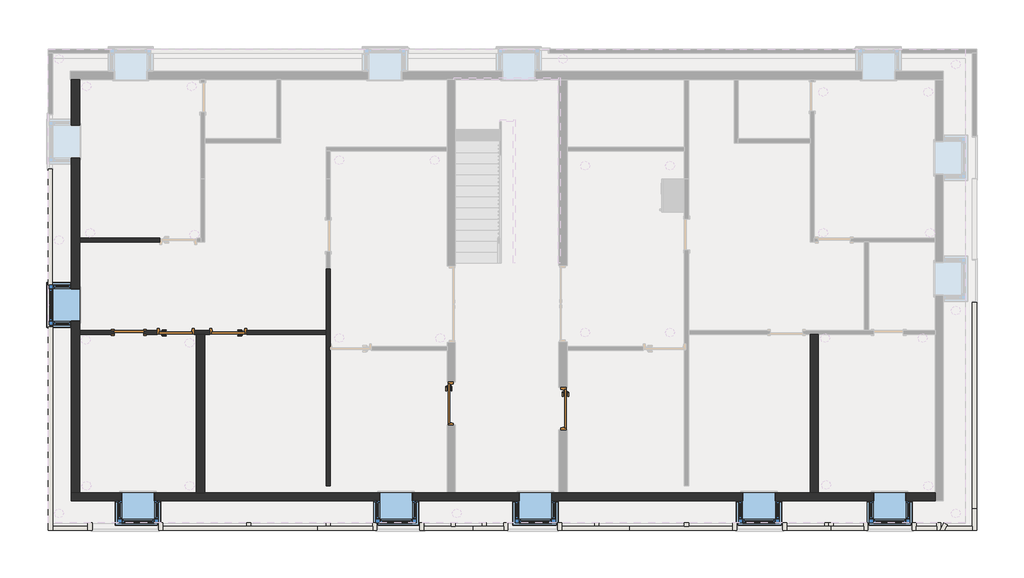
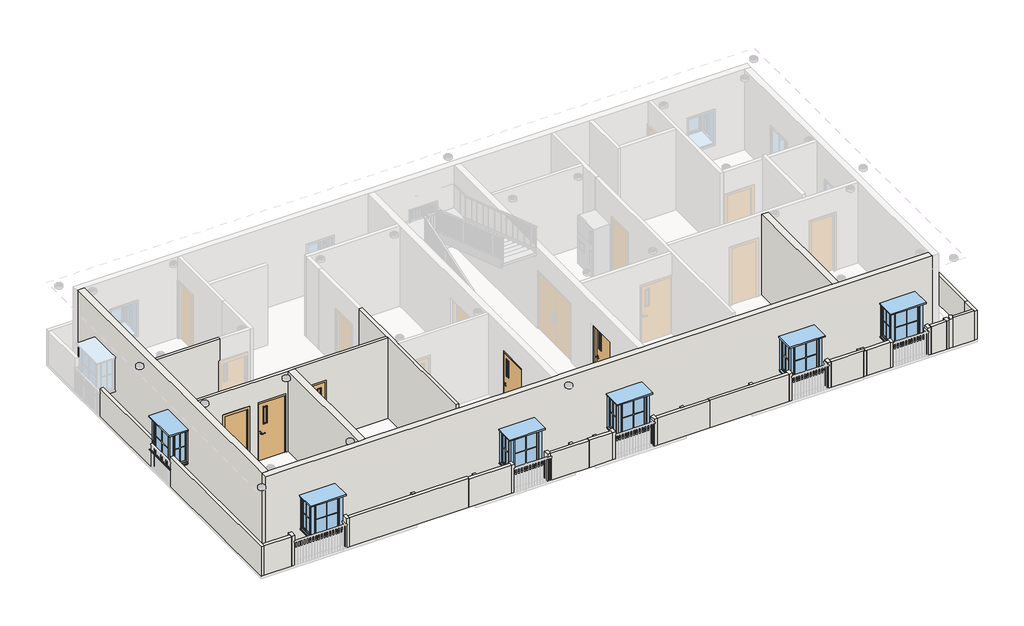
# One storey, part 1 of 7: 42 walls, 6 windows, 5 doors.
"""IFC4 building model written with IfcOpenShell, lengths in millimetres."""

from ifc_helpers import new_model, si_unit, frame, origin, place, context, project, spatial, polyline, outline, extrude, faceted_brep, transform, mapped, element, save
from components import door_586e558e, door_7d8f8091, door_passage_single_vision_lite_3_x7_440dd290, door_passage_single_vision_lite_3_x7_38248cdf, door_d141acb4, window_bay_casement_box_90_degree_angle_center_fixed_4_x3_2dea7aab

model = new_model("IFC4")

# Units and contexts
model_context = context("Model", 3, world=origin())
ifc_project = project(units=[si_unit("LENGTHUNIT", "METRE", prefix="MILLI")], contexts=[model_context])

# Site, building, storey
site = spatial("IfcSite", under=ifc_project)
building = spatial("IfcBuilding", under=site)
storey = spatial("IfcBuildingStorey", under=building, Elevation=3200.4)

# Doors
placement = place(None, origin())
door_shape = door_586e558e(model_context)
element("IfcDoor", 1, ObjectType="Door-Passage-Single-Vision_Lite : 3'6\"X7' 2", at=placement, inside=storey, context=model_context, shape_type="MappedRepresentation", body=[
    mapped(door_shape, transform((1116.1432011, -1461.3932193, 3200.4), x_axis=(0.0, -1.0, 0.0), y_axis=(1.0, 0.0, 0.0), z_axis=(0.0, 0.0, 1.0))),
])
door_2_shape = door_7d8f8091(model_context)
element("IfcDoor", 2, ObjectType="Door-Passage-Single-Vision_Lite : 3'7\"X7' 3", at=placement, inside=storey, context=model_context, shape_type="MappedRepresentation", body=[
    mapped(door_2_shape, transform((-1956.7487998, -1318.7421379, 3200.4), x_axis=(0.0, -1.0, 0.0), y_axis=(1.0, 0.0, 0.0), z_axis=(0.0, 0.0, 1.0))),
])
door_passage_single_vision_lite_3_x7_shape = door_passage_single_vision_lite_3_x7_440dd290(model_context)
element("IfcDoor", 3, ObjectType="Door-Passage-Single-Vision_Lite : 3'X7'", at=placement, inside=storey, context=model_context, shape_type="MappedRepresentation", body=[
    mapped(door_passage_single_vision_lite_3_x7_shape, transform((-8122.5987992, 646.8067334, 3200.4), x_axis=(-1.0, 0.0, 0.0), y_axis=(0.0, -1.0, 0.0), z_axis=(0.0, 0.0, 1.0))),
])
door_passage_single_vision_lite_3_x7_2_shape = door_passage_single_vision_lite_3_x7_38248cdf(model_context)
element("IfcDoor", 4, ObjectType="Door-Passage-Single-Vision_Lite : 3'X7'", at=placement, inside=storey, context=model_context, shape_type="MappedRepresentation", body=[
    mapped(door_passage_single_vision_lite_3_x7_2_shape, transform((-9570.3987992, 646.8067334, 3200.4), x_axis=(1.0, 0.0, 0.0), y_axis=(0.0, 1.0, 0.0), z_axis=(0.0, 0.0, 1.0))),
])
door_3_shape = door_d141acb4(model_context)
element("IfcDoor", 5, ObjectType="Single-Flush : 2'8\"x 7'", at=placement, inside=storey, context=model_context, shape_type="MappedRepresentation", body=[
    mapped(door_3_shape, transform((-10865.7987992, 640.4567334, 3200.4), x_axis=(1.0, 0.0, 0.0), y_axis=(0.0, 1.0, 0.0), z_axis=(0.0, 0.0, 1.0))),
])

# Walls
element("IfcWall", 6, ObjectType="Generic - 4.5\"", at=placement, inside=storey, context=model_context, shape_type="SweptSolid", body=[
    extrude(outline(polyline([(6248.4, -9959.0462614), (6248.4, -12224.6987925), (3200.4, -12224.6987925), (3200.4, -10009.8462614), (5435.6, -10009.8462614), (5435.6, -9959.0462614), (6248.4, -9959.0462614)])), frame((0.0, 3136.0067332, 0.0), z_axis=(0.0, 1.0, 0.0), x_axis=(0.0, 0.0, 1.0)), (0.0, 0.0, 1.0), 114.3),
])
element("IfcWall", 7, ObjectType="Generic - 4.5\"", at=placement, inside=storey, context=model_context, shape_type="Brep", body=[
    faceted_brep([(-10459.3987992, 583.3067334, 5334.0), (-10459.3987992, 583.3067334, 3200.4), (-10078.3987992, 583.3067334, 3200.4), (-10078.3987992, 583.3067334, 5435.6), (-9062.3987992, 583.3067334, 5435.6), (-9062.3987992, 583.3067334, 3200.4), (-8998.8987992, 583.3067334, 3200.4), (-8770.2987992, 583.3067334, 3200.4), (-8630.5987992, 583.3067334, 3200.4), (-8630.5987992, 583.3067334, 5435.6), (-7614.5987992, 583.3067334, 5435.6), (-7614.5987992, 583.3067334, 3200.4), (-5417.4987995, 583.3067334, 3200.4), (-5417.4987995, 583.3067334, 6248.4), (-8770.2987992, 583.3067334, 6248.4), (-8998.8987992, 583.3067334, 6248.4), (-12224.6987925, 583.3067334, 6248.4), (-12224.6987925, 583.3067334, 3200.4), (-11272.1987992, 583.3067334, 3200.4), (-11272.1987992, 583.3067334, 5334.0), (-10078.3987992, 697.6067334, 3200.4), (-10459.3987992, 697.6067334, 3200.4), (-10459.3987992, 697.6067334, 5334.0), (-11272.1987992, 697.6067334, 5334.0), (-11272.1987992, 697.6067334, 3200.4), (-12224.6987925, 697.6067334, 3200.4), (-12224.6987925, 697.6067334, 6248.4), (-5417.4987995, 697.6067334, 6248.4), (-5417.4987995, 697.6067334, 3200.4), (-7614.5987992, 697.6067334, 3200.4), (-7614.5987992, 697.6067334, 5435.6), (-8630.5987992, 697.6067334, 5435.6), (-8630.5987992, 697.6067334, 3200.4), (-9062.3987992, 697.6067334, 3200.4), (-9062.3987992, 697.6067334, 5435.6), (-10078.3987992, 697.6067334, 5435.6)], [[[0, 1, 2, 3, 4, 5, 6, 7, 8, 9, 10, 11, 12, 13, 14, 15, 16, 17, 18, 19]], [[20, 21, 22, 23, 24, 25, 26, 27, 28, 29, 30, 31, 32, 33, 34, 35]], [[28, 12, 11, 29]], [[32, 8, 7, 6, 5, 33]], [[18, 17, 25, 24]], [[2, 1, 21, 20]], [[16, 15, 14, 13, 27, 26]], [[17, 16, 26, 25]], [[13, 12, 28, 27]], [[9, 8, 32, 31]], [[10, 9, 31, 30]], [[11, 10, 30, 29]], [[4, 34, 33, 5]], [[34, 4, 3, 35]], [[35, 3, 2, 20]], [[22, 21, 1, 0]], [[23, 22, 0, 19]], [[24, 23, 19, 18]]]),
])
element("IfcWall", 8, ObjectType="Generic - 4.5\"", at=placement, inside=storey, context=model_context, shape_type="Brep", body=[
    faceted_brep([(-5417.4987995, 2399.4067802, 3200.4), (-5417.4987995, 697.6067334, 3200.4), (-5417.4987995, 583.3067334, 3200.4), (-5417.4987995, -3594.9932193, 3200.4), (-5417.4987995, -3594.9932193, 6248.4), (-5417.4987995, 583.3067334, 6248.4), (-5417.4987995, 697.6067334, 6248.4), (-5417.4987995, 2399.4067802, 6248.4), (-5303.1987995, -3594.9932193, 6248.4), (-5303.1987995, -3594.9932193, 3200.4), (-5303.1987995, 148.1078621, 3200.4), (-5303.1987995, 148.1078621, 5435.6), (-5303.1987995, 262.4078621, 5435.6), (-5303.1987995, 262.4078621, 3200.4), (-5303.1987995, 2399.4067802, 3200.4), (-5303.1987995, 2399.4067802, 6248.4), (-5303.1987995, 262.4078621, 6248.4), (-5303.1987995, 148.1078621, 6248.4), (-5334.9487995, 262.4078621, 3200.4), (-5334.9487995, 148.1078621, 3200.4), (-5334.9487995, 262.4078621, 5435.6), (-5334.9487995, 148.1078621, 5435.6)], [[[0, 1, 2, 3, 4, 5, 6, 7]], [[8, 9, 10, 11, 12, 13, 14, 15, 16, 17]], [[3, 2, 1, 0, 14, 13, 18, 19, 10, 9]], [[4, 3, 9, 8]], [[7, 6, 5, 4, 8, 17, 16, 15]], [[0, 7, 15, 14]], [[20, 18, 13, 12]], [[19, 21, 11, 10]], [[21, 20, 12, 11]], [[18, 20, 21, 19]]]),
])
element("IfcWall", 9, ObjectType="Generic - 4.5\"", at=placement, inside=storey, context=model_context, shape_type="SweptSolid", body=[
    extrude(outline(polyline([(-11996.6067989, -4826.8932661), (-12974.5067989, -4826.8932661), (-12974.5067989, -4712.5932661), (-11996.6067989, -4712.5932661), (-11996.6067989, -4826.8932661)])), frame((0.0, 0.0, 3200.4), z_axis=(0.0, 0.0, 1.0), x_axis=(1.0, 0.0, 0.0)), (0.0, 0.0, 1.0), 1112.9417562),
])
element("IfcWall", 10, ObjectType="Generic - 4.5\"", at=placement, inside=storey, context=model_context, shape_type="Brep", body=[
    faceted_brep([(-13088.8067989, 792.8567339, 3200.4), (-13088.8067989, -4826.8932661, 3200.4), (-13088.8067989, -4826.8932661, 4314.567936), (-13088.8067989, 792.8567339, 4314.567936), (-12974.5067989, 792.8567339, 3200.4), (-12974.5067989, 792.8567339, 4314.567936), (-12974.5067989, -4826.8932661, 4314.567936), (-12974.5067989, -4826.8932661, 4313.3417562), (-12974.5067989, -4826.8932661, 3200.4), (-12974.5067989, -4712.5932661, 3200.4)], [[[0, 1, 2, 3]], [[4, 5, 6, 7, 8, 9]], [[1, 0, 4, 9, 8]], [[3, 2, 6, 5]], [[0, 3, 5, 4]], [[2, 1, 8, 7, 6]]]),
])
element("IfcWall", 11, ObjectType="Generic - 4.5\"", at=placement, inside=storey, context=model_context, shape_type="Brep", body=[
    faceted_brep([(-11996.6067989, -4623.6932193, 3200.4), (-11996.6067989, -4712.5932661, 3200.4), (-11996.6067989, -4826.8932661, 3200.4), (-11996.6067989, -4826.8932661, 4313.3417562), (-11996.6067989, -4826.8932661, 4334.3303619), (-11996.6067989, -4623.6932193, 4334.3303619), (-11882.3067989, -4623.6932193, 3200.4), (-11882.3067989, -4623.6932193, 4334.3303619), (-11882.3067989, -4826.8932661, 4334.3303619), (-11882.3067989, -4826.8932661, 3200.4)], [[[0, 1, 2, 3, 4, 5]], [[6, 7, 8, 9]], [[2, 1, 0, 6, 9]], [[5, 4, 8, 7]], [[0, 5, 7, 6]], [[4, 3, 2, 9, 8]]]),
])
element("IfcWall", 12, ObjectType="Generic - 4.5\"", at=placement, inside=storey, context=model_context, shape_type="Brep", body=[
    faceted_brep([(11660.3143245, -4826.8932661, 3200.4), (12426.0012043, -4826.8932661, 3200.4), (12426.0012043, -4826.8932661, 4292.2617784), (12426.0012043, -4826.8932661, 4303.5196614), (11660.3143245, -4826.8932661, 4303.5196614), (11660.3143245, -4826.8932661, 4289.9342527), (11716.0621594, -4712.5932661, 3200.4), (11716.0621594, -4712.5932661, 4303.5196614), (12426.0012043, -4712.5932661, 4303.5196614), (12426.0012043, -4712.5932661, 3200.4)], [[[0, 1, 2, 3, 4, 5]], [[6, 7, 8, 9]], [[1, 0, 6, 9]], [[4, 3, 8, 7]], [[3, 2, 1, 9, 8]], [[0, 5, 4, 7, 6]]]),
])
element("IfcWall", 13, ObjectType="Generic - 4.5\"", at=placement, inside=storey, context=model_context, shape_type="Brep", body=[
    faceted_brep([(11632.2512075, -4623.6932193, 3200.4), (11533.1439227, -4826.8932661, 3200.4), (11533.1439227, -4826.8932661, 4289.9342527), (11632.2512075, -4623.6932193, 4289.9342527), (11734.983367, -4673.7990414, 3200.4), (11734.983367, -4673.7990414, 4289.9342527), (11660.3143245, -4826.8932661, 4289.9342527), (11660.3143245, -4826.8932661, 3200.4), (11716.0621594, -4712.5932661, 3200.4)], [[[0, 1, 2, 3]], [[4, 5, 6, 7, 8]], [[1, 0, 4, 8, 7]], [[3, 2, 6, 5]], [[0, 3, 5, 4]], [[2, 1, 7, 6]]]),
])
element("IfcWall", 14, ObjectType="Generic - 4.5\"", at=placement, inside=storey, context=model_context, shape_type="Brep", body=[
    faceted_brep([(12426.0012043, -4236.3432661, 3200.4), (12426.0012043, -4712.5932661, 3200.4), (12426.0012043, -4826.8932661, 3200.4), (12426.0012043, -4826.8932661, 4292.2617784), (12426.0012043, -4236.3432661, 4292.2617784), (12426.0012043, -4236.3432661, 4287.0712164), (12540.3012043, -4236.3432661, 3200.4), (12540.3012043, -4236.3432661, 4287.0712164), (12540.3012043, -4236.3432661, 4292.2617784), (12540.3012043, -4826.8932661, 4292.2617784), (12540.3012043, -4826.8932661, 3200.4)], [[[0, 1, 2, 3, 4, 5]], [[6, 7, 8, 9, 10]], [[2, 1, 0, 6, 10]], [[4, 3, 9, 8]], [[0, 5, 4, 8, 7, 6]], [[3, 2, 10, 9]]]),
])
element("IfcWall", 15, ObjectType="Generic - 4.5\"", at=placement, inside=storey, context=model_context, shape_type="SweptSolid", body=[
    extrude(outline(polyline([(-5417.4987995, -4712.5932661), (-5417.4987995, -4623.6932193), (-5303.1987995, -4623.6932193), (-5303.1987995, -4712.5932661), (-5417.4987995, -4712.5932661)])), frame((0.0, 0.0, 3200.4), z_axis=(0.0, 0.0, 1.0), x_axis=(1.0, 0.0, 0.0)), (0.0, 0.0, 1.0), 1063.0786215),
])
element("IfcWall", 16, ObjectType="Generic - 4.5\"", at=placement, inside=storey, context=model_context, shape_type="Brep", body=[
    faceted_brep([(-5663.8033402, -4826.8932661, 3200.4), (-4134.7987995, -4826.8932661, 3200.4), (-4134.7987995, -4826.8932661, 4259.5218247), (-4134.7987995, -4826.8932661, 4267.6575049), (-5663.8033402, -4826.8932661, 4267.6575049), (-5663.8033402, -4712.5932661, 3200.4), (-5663.8033402, -4712.5932661, 4267.6575049), (-4134.7987995, -4712.5932661, 4267.6575049), (-4134.7987995, -4712.5932661, 3200.4), (-5303.1987995, -4712.5932661, 3200.4), (-5417.4987995, -4712.5932661, 3200.4)], [[[0, 1, 2, 3, 4]], [[5, 6, 7, 8, 9, 10]], [[1, 0, 5, 10, 9, 8]], [[4, 3, 7, 6]], [[0, 4, 6, 5]], [[3, 2, 1, 8, 7]]]),
])
element("IfcWall", 17, ObjectType="Generic - 4.5\"", at=placement, inside=storey, context=model_context, shape_type="Brep", body=[
    faceted_brep([(-2725.0987995, -4826.8932661, 3200.4), (-1354.4417672, -4826.8932661, 3200.4), (-1354.4417672, -4826.8932661, 4216.4), (-2725.0987995, -4826.8932661, 4216.4), (-2725.0987995, -4712.5932661, 3200.4), (-2725.0987995, -4712.5932661, 4216.4), (-1354.4417672, -4712.5932661, 4216.4), (-1354.4417672, -4712.5932661, 3200.4), (-1848.7987998, -4712.5932661, 3200.4), (-1963.0987998, -4712.5932661, 3200.4)], [[[0, 1, 2, 3]], [[4, 5, 6, 7, 8, 9]], [[1, 0, 4, 9, 8, 7]], [[2, 1, 7, 6]], [[3, 2, 6, 5]], [[0, 3, 5, 4]]]),
])
element("IfcWall", 18, ObjectType="Generic - 4.5\"", at=placement, inside=storey, context=model_context, shape_type="SweptSolid", body=[
    extrude(outline(polyline([(-1963.0987998, -4712.5932661), (-1963.0987998, -4623.6932193), (-1848.7987998, -4623.6932193), (-1848.7987998, -4712.5932661), (-1963.0987998, -4712.5932661)])), frame((0.0, 0.0, 3200.4), z_axis=(0.0, 0.0, 1.0), x_axis=(1.0, 0.0, 0.0)), (0.0, 0.0, 1.0), 1029.3234006),
])
element("IfcWall", 19, ObjectType="Generic - 4.5\"", at=placement, inside=storey, context=model_context, shape_type="SweptSolid", body=[
    extrude(outline(polyline([(-1112.1987998, -4712.5932661), (-1112.1987998, -4623.6932193), (-997.8987998, -4623.6932193), (-997.8987998, -4712.5932661), (-1112.1987998, -4712.5932661)])), frame((0.0, 0.0, 3200.4), z_axis=(0.0, 0.0, 1.0), x_axis=(1.0, 0.0, 0.0)), (0.0, 0.0, 1.0), 1016.0),
])
element("IfcWall", 20, ObjectType="Generic - 4.5\"", at=placement, inside=storey, context=model_context, shape_type="SweptSolid", body=[
    extrude(outline(polyline([(1999.3012002, -4712.5932661), (1999.3012002, -4623.6932193), (2113.6012002, -4623.6932193), (2113.6012002, -4712.5932661), (1999.3012002, -4712.5932661)])), frame((0.0, 0.0, 3200.4), z_axis=(0.0, 0.0, 1.0), x_axis=(1.0, 0.0, 0.0)), (0.0, 0.0, 1.0), 1013.2250283),
])
element("IfcWall", 21, ObjectType="Generic - 4.5\"", at=placement, inside=storey, context=model_context, shape_type="SweptSolid", body=[
    extrude(outline(polyline([(4475.8012082, -4712.5932661), (4475.8012082, -4623.6932193), (4590.1012082, -4623.6932193), (4590.1012082, -4712.5932661), (4475.8012082, -4712.5932661)])), frame((0.0, 0.0, 3200.4), z_axis=(0.0, 0.0, 1.0), x_axis=(1.0, 0.0, 0.0)), (0.0, 0.0, 1.0), 1027.4591445),
])
element("IfcWall", 22, ObjectType="Generic - 4.5\"", at=placement, inside=storey, context=model_context, shape_type="Brep", body=[
    faceted_brep([(2962.6087812, -4826.8932661, 3200.4), (5802.9512082, -4826.8932661, 3200.4), (5802.9512082, -4826.8932661, 4227.8591445), (2962.6087812, -4826.8932661, 4227.8591445), (2962.6087812, -4826.8932661, 4213.6250283), (2962.6087812, -4712.5932661, 3200.4), (2962.6087812, -4712.5932661, 4213.6250283), (2962.6087812, -4712.5932661, 4227.8591445), (4475.8012082, -4712.5932661, 4227.8591445), (4590.1012082, -4712.5932661, 4227.8591445), (5802.9512082, -4712.5932661, 4227.8591445), (5802.9512082, -4712.5932661, 3200.4), (4590.1012082, -4712.5932661, 3200.4), (4475.8012082, -4712.5932661, 3200.4)], [[[0, 1, 2, 3, 4]], [[5, 6, 7, 8, 9, 10, 11, 12, 13]], [[1, 0, 5, 13, 12, 11]], [[3, 2, 10, 9, 8, 7]], [[0, 4, 3, 7, 6, 5]], [[2, 1, 11, 10]]]),
])
element("IfcWall", 23, ObjectType="Generic - 4.5\"", at=placement, inside=storey, context=model_context, shape_type="Brep", body=[
    faceted_brep([(5802.9512082, -4623.6932193, 3200.4), (5802.9512082, -4712.5932661, 3200.4), (5802.9512082, -4826.8932661, 3200.4), (5802.9512082, -4826.8932661, 4227.8591445), (5802.9512082, -4826.8932661, 4232.7822201), (5802.9512082, -4623.6932193, 4232.7822201), (5917.2512082, -4623.6932193, 3200.4), (5917.2512082, -4623.6932193, 4232.7822201), (5917.2512082, -4826.8932661, 4232.7822201), (5917.2512082, -4826.8932661, 3200.4)], [[[0, 1, 2, 3, 4, 5]], [[6, 7, 8, 9]], [[2, 1, 0, 6, 9]], [[5, 4, 8, 7]], [[0, 5, 7, 6]], [[4, 3, 2, 9, 8]]]),
])
element("IfcWall", 24, ObjectType="Generic - 4.5\"", at=placement, inside=storey, context=model_context, shape_type="Brep", body=[
    faceted_brep([(7190.3011643, -4623.6932193, 3200.4), (7190.3011643, -4826.8932661, 3200.4), (7190.3011643, -4826.8932661, 4173.2158009), (7190.3011643, -4623.6932193, 4173.2158009), (7304.6011643, -4623.6932193, 3200.4), (7304.6011643, -4623.6932193, 4173.2158009), (7304.6011643, -4712.5932661, 4173.2158009), (7304.6011643, -4826.8932661, 4173.2158009), (7304.6011643, -4826.8932661, 3200.4), (7304.6011643, -4712.5932661, 3200.4)], [[[0, 1, 2, 3]], [[4, 5, 6, 7, 8, 9]], [[1, 0, 4, 9, 8]], [[3, 2, 7, 6, 5]], [[0, 3, 5, 4]], [[2, 1, 8, 7]]]),
])
element("IfcWall", 25, ObjectType="Generic - 4.5\"", at=placement, inside=storey, context=model_context, shape_type="Brep", body=[
    faceted_brep([(7304.6011643, -4826.8932661, 3200.4), (8463.6012082, -4826.8932661, 3200.4), (8463.6012082, -4826.8932661, 4156.8159658), (8520.7512082, -4826.8932661, 4156.8159658), (8520.7512082, -4826.8932661, 4170.080309), (8520.7512082, -4826.8932661, 4173.3581334), (7304.6011643, -4826.8932661, 4173.3581334), (7304.6011643, -4712.5932661, 3200.4), (7304.6011643, -4712.5932661, 4173.3581334), (8520.7512082, -4712.5932661, 4173.3581334), (8520.7512082, -4712.5932661, 4170.080309), (8520.7512082, -4712.5932661, 4156.8159658), (8463.6012082, -4712.5932661, 4156.8159658), (8463.6012082, -4712.5932661, 3200.4), (8457.2512082, -4712.5932661, 3200.4), (8342.9512082, -4712.5932661, 3200.4)], [[[0, 1, 2, 3, 4, 5, 6]], [[7, 8, 9, 10, 11, 12, 13, 14, 15]], [[1, 0, 7, 15, 14, 13]], [[6, 5, 9, 8]], [[0, 6, 8, 7]], [[5, 4, 3, 11, 10, 9]], [[11, 3, 2, 12]], [[2, 1, 13, 12]]]),
])
element("IfcWall", 26, ObjectType="Generic - 4.5\"", at=placement, inside=storey, context=model_context, shape_type="SweptSolid", body=[
    extrude(outline(polyline([(8342.9512082, -4712.5932661), (8342.9512082, -4623.6932193), (8457.2512082, -4623.6932193), (8457.2512082, -4712.5932661), (8342.9512082, -4712.5932661)])), frame((0.0, 0.0, 3200.4), z_axis=(0.0, 0.0, 1.0), x_axis=(1.0, 0.0, 0.0)), (0.0, 0.0, 1.0), 954.7500484),
])
element("IfcWall", 27, ObjectType="Generic - 4.5\"", at=placement, inside=storey, context=model_context, shape_type="Brep", body=[
    faceted_brep([(8463.6012082, -4623.6932193, 3200.4), (8463.6012082, -4712.5932661, 3200.4), (8463.6012082, -4826.8932661, 3200.4), (8463.6012082, -4826.8932661, 4156.8159658), (8463.6012082, -4712.5932661, 4156.8159658), (8463.6012082, -4623.6932193, 4156.8159658), (8577.9012082, -4623.6932193, 3200.4), (8577.9012082, -4623.6932193, 4156.8159658), (8577.9012082, -4712.5932661, 4156.8159658), (8577.9012082, -4826.8932661, 4156.8159658), (8577.9012082, -4826.8932661, 3200.4), (8577.9012082, -4712.5932661, 3200.4), (8520.7512082, -4826.8932661, 4156.8159658)], [[[0, 1, 2, 3, 4, 5]], [[6, 7, 8, 9, 10, 11]], [[2, 1, 0, 6, 11, 10]], [[5, 4, 3, 12, 9, 8, 7]], [[0, 5, 7, 6]], [[3, 2, 10, 9, 12]]]),
])
element("IfcWall", 28, ObjectType="Generic - 4.5\"", at=placement, inside=storey, context=model_context, shape_type="Brep", body=[
    faceted_brep([(8577.9012082, -4826.8932661, 3200.4), (9422.4512082, -4826.8932661, 3200.4), (9422.4512082, -4826.8932661, 4152.6060641), (9422.4512082, -4826.8932661, 4170.080309), (8520.7512082, -4826.8932661, 4170.080309), (8520.7512082, -4826.8932661, 4156.8159658), (8577.9012082, -4826.8932661, 4156.8159658), (8577.9012082, -4712.5932661, 3200.4), (8577.9012082, -4712.5932661, 4156.8159658), (8520.7512082, -4712.5932661, 4156.8159658), (8520.7512082, -4712.5932661, 4170.080309), (9422.4512082, -4712.5932661, 4170.080309), (9422.4512082, -4712.5932661, 3200.4)], [[[0, 1, 2, 3, 4, 5, 6]], [[7, 8, 9, 10, 11, 12]], [[1, 0, 7, 12]], [[4, 3, 11, 10]], [[3, 2, 1, 12, 11]], [[5, 4, 10, 9]], [[5, 9, 8, 6]], [[0, 6, 8, 7]]]),
])
element("IfcWall", 29, ObjectType="Generic - 4.5\"", at=placement, inside=storey, context=model_context, shape_type="Brep", body=[
    faceted_brep([(9422.4512082, -4623.6932193, 3200.4), (9422.4512082, -4712.5932661, 3200.4), (9422.4512082, -4826.8932661, 3200.4), (9422.4512082, -4826.8932661, 4152.6060641), (9422.4512082, -4623.6932193, 4152.6060641), (9536.7512082, -4623.6932193, 3200.4), (9536.7512082, -4623.6932193, 4152.6060641), (9536.7512082, -4826.8932661, 4152.6060641), (9536.7512082, -4826.8932661, 3200.4)], [[[0, 1, 2, 3, 4]], [[5, 6, 7, 8]], [[2, 1, 0, 5, 8]], [[4, 3, 7, 6]], [[0, 4, 6, 5]], [[3, 2, 8, 7]]]),
])
element("IfcWall", 30, ObjectType="Generic - 4.5\"", at=placement, inside=storey, context=model_context, shape_type="Brep", body=[
    faceted_brep([(10764.1617205, -4623.6932193, 3200.4), (10764.1617205, -4826.8932661, 3200.4), (10764.1617205, -4826.8932661, 4226.7072304), (10764.1617205, -4623.6932193, 4226.7072304), (10878.4617205, -4623.6932193, 3200.4), (10878.4617205, -4623.6932193, 4226.7072304), (10878.4617205, -4826.8932661, 4226.7072304), (10878.4617205, -4826.8932661, 3200.4), (10878.4617205, -4712.5932661, 3200.4)], [[[0, 1, 2, 3]], [[4, 5, 6, 7, 8]], [[1, 0, 4, 8, 7]], [[3, 2, 6, 5]], [[0, 3, 5, 4]], [[2, 1, 7, 6]]]),
])
element("IfcWall", 31, ObjectType="Generic - 4.5\"", at=placement, inside=storey, context=model_context, shape_type="Brep", body=[
    faceted_brep([(10878.4617205, -4826.8932661, 3200.4), (11437.2617205, -4826.8932661, 3200.4), (11437.2617205, -4826.8932661, 4249.0912221), (10878.4617205, -4826.8932661, 4249.0912221), (10878.4617205, -4826.8932661, 4226.7072304), (10878.4617205, -4712.5932661, 3200.4), (10878.4617205, -4712.5932661, 4249.0912221), (11437.2617205, -4712.5932661, 4249.0912221), (11437.2617205, -4712.5932661, 3200.4)], [[[0, 1, 2, 3, 4]], [[5, 6, 7, 8]], [[1, 0, 5, 8]], [[3, 2, 7, 6]], [[0, 4, 3, 6, 5]], [[2, 1, 8, 7]]]),
])
element("IfcWall", 32, ObjectType="Generic - 4.5\"", at=placement, inside=storey, context=model_context, shape_type="Brep", body=[
    faceted_brep([(11437.2617205, -4623.6932193, 3200.4), (11437.2617205, -4712.5932661, 3200.4), (11437.2617205, -4826.8932661, 3200.4), (11437.2617205, -4826.8932661, 4249.0912221), (11437.2617205, -4712.5932661, 4249.0912221), (11437.2617205, -4623.6932193, 4249.0912221), (11551.5617205, -4623.6932193, 3200.4), (11551.5617205, -4623.6932193, 4249.0912221), (11551.5617205, -4826.8932661, 4249.0912221), (11551.5617205, -4826.8932661, 3200.4)], [[[0, 1, 2, 3, 4, 5]], [[6, 7, 8, 9]], [[2, 1, 0, 6, 9]], [[5, 4, 3, 8, 7]], [[0, 5, 7, 6]], [[3, 2, 9, 8]]]),
])
element("IfcWall", 33, ObjectType="Generic - 4.5\"", at=placement, inside=storey, context=model_context, shape_type="Brep", body=[
    faceted_brep([(-4134.7987995, -4623.6932193, 3200.4), (-4134.7987995, -4712.5932661, 3200.4), (-4134.7987995, -4826.8932661, 3200.4), (-4134.7987995, -4826.8932661, 4259.5218247), (-4134.7987995, -4623.6932193, 4259.5218247), (-4020.4987995, -4623.6932193, 3200.4), (-4020.4987995, -4623.6932193, 4259.5218247), (-4020.4987995, -4826.8932661, 4259.5218247), (-4020.4987995, -4826.8932661, 3200.4)], [[[0, 1, 2, 3, 4]], [[5, 6, 7, 8]], [[2, 1, 0, 5, 8]], [[4, 3, 7, 6]], [[0, 4, 6, 5]], [[3, 2, 8, 7]]]),
])
element("IfcWall", 34, ObjectType="Generic - 4.5\"", at=placement, inside=storey, context=model_context, shape_type="Brep", body=[
    faceted_brep([(-2839.3987995, -4623.6932193, 3200.4), (-2839.3987995, -4826.8932661, 3200.4), (-2839.3987995, -4826.8932661, 4217.1549618), (-2839.3987995, -4623.6932193, 4217.1549618), (-2725.0987995, -4623.6932193, 3200.4), (-2725.0987995, -4623.6932193, 4217.1549618), (-2725.0987995, -4826.8932661, 4217.1549618), (-2725.0987995, -4826.8932661, 4216.4), (-2725.0987995, -4826.8932661, 3200.4), (-2725.0987995, -4712.5932661, 3200.4)], [[[0, 1, 2, 3]], [[4, 5, 6, 7, 8, 9]], [[1, 0, 4, 9, 8]], [[3, 2, 6, 5]], [[0, 3, 5, 4]], [[2, 1, 8, 7, 6]]]),
])
element("IfcWall", 35, ObjectType="Generic - 4.5\"", at=placement, inside=storey, context=model_context, shape_type="Brep", body=[
    faceted_brep([(-1354.4417672, -4826.8932661, 3200.4), (-520.5065315, -4826.8932661, 3200.4), (-520.5065315, -4826.8932661, 4224.2796817), (-520.5065315, -4826.8932661, 4231.540074), (-1354.4417672, -4826.8932661, 4231.540074), (-1354.4417672, -4826.8932661, 4216.4), (-1354.4417672, -4712.5932661, 3200.4), (-1354.4417672, -4712.5932661, 4216.4), (-1354.4417672, -4712.5932661, 4231.540074), (-520.5065315, -4712.5932661, 4231.540074), (-520.5065315, -4712.5932661, 3200.4), (-997.8987998, -4712.5932661, 3200.4), (-1112.1987998, -4712.5932661, 3200.4)], [[[0, 1, 2, 3, 4, 5]], [[6, 7, 8, 9, 10, 11, 12]], [[1, 0, 6, 12, 11, 10]], [[4, 3, 9, 8]], [[0, 5, 4, 8, 7, 6]], [[3, 2, 1, 10, 9]]]),
])
element("IfcWall", 36, ObjectType="Generic - 4.5\"", at=placement, inside=storey, context=model_context, shape_type="Brep", body=[
    faceted_brep([(-520.5065315, -4623.6932193, 3200.4), (-520.5065315, -4712.5932661, 3200.4), (-520.5065315, -4826.8932661, 3200.4), (-520.5065315, -4826.8932661, 4224.2796817), (-520.5065315, -4623.6932193, 4224.2796817), (-406.2065315, -4623.6932193, 3200.4), (-406.2065315, -4623.6932193, 4224.2796817), (-406.2065315, -4826.8932661, 4224.2796817), (-406.2065315, -4826.8932661, 3200.4)], [[[0, 1, 2, 3, 4]], [[5, 6, 7, 8]], [[2, 1, 0, 5, 8]], [[4, 3, 7, 6]], [[0, 4, 6, 5]], [[3, 2, 8, 7]]]),
])
element("IfcWall", 37, ObjectType="Generic - 4.5\"", at=placement, inside=storey, context=model_context, shape_type="Brep", body=[
    faceted_brep([(970.0932011, -4623.6932193, 3200.4), (970.0932011, -4826.8932661, 3200.4), (970.0932011, -4826.8932661, 4213.6250283), (970.0932011, -4623.6932193, 4213.6250283), (1084.3932011, -4623.6932193, 3200.4), (1084.3932011, -4623.6932193, 4213.6250283), (1084.3932011, -4712.5932661, 4213.6250283), (1084.3932011, -4826.8932661, 4213.6250283), (1084.3932011, -4826.8932661, 3200.4), (1084.3932011, -4712.5932661, 3200.4)], [[[0, 1, 2, 3]], [[4, 5, 6, 7, 8, 9]], [[1, 0, 4, 9, 8]], [[3, 2, 7, 6, 5]], [[0, 3, 5, 4]], [[2, 1, 8, 7]]]),
])
element("IfcWall", 38, ObjectType="Generic - 4.5\"", at=placement, inside=storey, context=model_context, shape_type="Brep", body=[
    faceted_brep([(1084.3932011, -4826.8932661, 3200.4), (2962.6087812, -4826.8932661, 3200.4), (2962.6087812, -4826.8932661, 4213.6250283), (1084.3932011, -4826.8932661, 4213.6250283), (1084.3932011, -4712.5932661, 3200.4), (1084.3932011, -4712.5932661, 4213.6250283), (1999.3012002, -4712.5932661, 4213.6250283), (2113.6012002, -4712.5932661, 4213.6250283), (2962.6087812, -4712.5932661, 4213.6250283), (2962.6087812, -4712.5932661, 3200.4), (2113.6012002, -4712.5932661, 3200.4), (1999.3012002, -4712.5932661, 3200.4)], [[[0, 1, 2, 3]], [[4, 5, 6, 7, 8, 9, 10, 11]], [[1, 0, 4, 11, 10, 9]], [[2, 1, 9, 8]], [[3, 2, 8, 7, 6, 5]], [[0, 3, 5, 4]]]),
])
element("IfcWall", 39, ObjectType="Generic - 4.5\"", at=placement, inside=storey, context=model_context, shape_type="Brep", body=[
    faceted_brep([(-10045.9470335, -4623.6932193, 3200.4), (-10045.9470335, -4826.8932661, 3200.4), (-10045.9470335, -4826.8932661, 4308.104535), (-10045.9470335, -4623.6932193, 4308.104535), (-9931.6470335, -4623.6932193, 3200.4), (-9931.6470335, -4623.6932193, 4308.104535), (-9931.6470335, -4712.5932661, 4308.104535), (-9931.6470335, -4826.8932661, 4308.104535), (-9931.6470335, -4826.8932661, 3200.4), (-9931.6470335, -4712.5932661, 3200.4)], [[[0, 1, 2, 3]], [[4, 5, 6, 7, 8, 9]], [[1, 0, 4, 9, 8]], [[3, 2, 7, 6, 5]], [[0, 3, 5, 4]], [[2, 1, 8, 7]]]),
])
element("IfcWall", 40, ObjectType="Generic - 4.5\"", at=placement, inside=storey, context=model_context, shape_type="Brep", body=[
    faceted_brep([(-9931.6470335, -4826.8932661, 3200.4), (-5663.8033402, -4826.8932661, 3200.4), (-5663.8033402, -4826.8932661, 4267.6575049), (-5663.8033402, -4826.8932661, 4308.104535), (-9931.6470335, -4826.8932661, 4308.104535), (-9931.6470335, -4712.5932661, 3200.4), (-9931.6470335, -4712.5932661, 4308.104535), (-7614.8527957, -4712.5932661, 4308.104535), (-7500.5527957, -4712.5932661, 4308.104535), (-5663.8033402, -4712.5932661, 4308.104535), (-5663.8033402, -4712.5932661, 4267.6575049), (-5663.8033402, -4712.5932661, 3200.4), (-7500.5527957, -4712.5932661, 3200.4), (-7614.8527957, -4712.5932661, 3200.4)], [[[0, 1, 2, 3, 4]], [[5, 6, 7, 8, 9, 10, 11, 12, 13]], [[1, 0, 5, 13, 12, 11]], [[3, 2, 1, 11, 10, 9]], [[4, 3, 9, 8, 7, 6]], [[0, 4, 6, 5]]]),
])
element("IfcWall", 41, ObjectType="Generic - 4.5\"", at=placement, inside=storey, context=model_context, shape_type="SweptSolid", body=[
    extrude(outline(polyline([(-7614.8527957, -4712.5932661), (-7614.8527957, -4623.6932193), (-7500.5527957, -4623.6932193), (-7500.5527957, -4712.5932661), (-7614.8527957, -4712.5932661)])), frame((0.0, 0.0, 3200.4), z_axis=(0.0, 0.0, 1.0), x_axis=(1.0, 0.0, 0.0)), (0.0, 0.0, 1.0), 1107.704535),
])
element("IfcWall", 42, ObjectType="Generic - 4.5\"", at=placement, inside=storey, context=model_context, shape_type="SweptSolid", body=[
    extrude(outline(polyline([(-12976.0338648, 5154.3604213), (-12976.0338648, 1953.9604213), (-13090.3338648, 1953.9604213), (-13090.3338648, 5154.3604213), (-12976.0338648, 5154.3604213)])), frame((0.0, 0.0, 3200.4), z_axis=(0.0, 0.0, 1.0), x_axis=(1.0, 0.0, 0.0)), (0.0, 0.0, 1.0), 1047.4413329),
])
element("IfcWall", 43, ObjectType="Generic - 4.5\"", at=placement, inside=storey, context=model_context, shape_type="SweptSolid", body=[
    extrude(outline(polyline([(12426.0012043, -4236.3432661), (12426.0012043, 1478.6567334), (12540.3012043, 1478.6567334), (12540.3012043, -4236.3432661), (12426.0012043, -4236.3432661)])), frame((0.0, 0.0, 3200.4), z_axis=(0.0, 0.0, 1.0), x_axis=(1.0, 0.0, 0.0)), (0.0, 0.0, 1.0), 1086.6712164),
])
element("IfcWall", 44, ObjectType="Generic - 9\"", at=placement, inside=storey, context=model_context, shape_type="Brep", body=[
    faceted_brep([(11397.3012075, -3785.4932193, 3200.4), (8171.5012079, -3785.4932193, 3200.4), (7942.9012079, -3785.4932193, 3200.4), (1236.7932011, -3785.4932193, 3200.4), (1008.1932011, -3785.4932193, 3200.4), (-1848.7987998, -3785.4932193, 3200.4), (-2077.3987998, -3785.4932193, 3200.4), (-8770.2987992, -3785.4932193, 3200.4), (-8998.8987992, -3785.4932193, 3200.4), (-12224.6987925, -3785.4932193, 3200.4), (-12453.2987925, -3785.4932193, 3200.4), (-12453.2987925, -3785.4932193, 6248.4), (-12224.6987925, -3785.4932193, 6248.4), (-8998.8987992, -3785.4932193, 6248.4), (-8770.2987992, -3785.4932193, 6248.4), (-2077.3987998, -3785.4932193, 6248.4), (-1848.7987998, -3785.4932193, 6248.4), (1008.1932011, -3785.4932193, 6248.4), (1236.7932011, -3785.4932193, 6248.4), (7942.9012079, -3785.4932193, 6248.4), (8171.5012079, -3785.4932193, 6248.4), (11397.3012075, -3785.4932193, 6248.4), (-11068.9987958, -3785.4932193, 5080.0), (-11068.9987958, -3785.4932193, 3810.0), (-10154.5987958, -3785.4932193, 3810.0), (-10154.5987958, -3785.4932193, 5080.0), (-3944.2987998, -3785.4932193, 5080.0), (-3944.2987998, -3785.4932193, 3810.0), (-3029.8987998, -3785.4932193, 3810.0), (-3029.8987998, -3785.4932193, 5080.0), (-96.7067989, -3785.4932193, 5080.0), (-96.7067989, -3785.4932193, 3810.0), (817.6932011, -3785.4932193, 3810.0), (817.6932011, -3785.4932193, 5080.0), (6076.0012079, -3785.4932193, 5080.0), (6076.0012079, -3785.4932193, 3810.0), (6990.4012079, -3785.4932193, 3810.0), (6990.4012079, -3785.4932193, 5080.0), (9682.8012075, -3785.4932193, 5080.0), (9682.8012075, -3785.4932193, 3810.0), (10597.2012075, -3785.4932193, 3810.0), (10597.2012075, -3785.4932193, 5080.0), (11397.3012075, -4014.0932193, 3200.4), (11397.3012075, -4014.0932193, 6248.4), (-12453.2987925, -4014.0932193, 6248.4), (-12453.2987925, -4014.0932193, 3200.4), (-11068.9987958, -4014.0932193, 5080.0), (-10154.5987958, -4014.0932193, 5080.0), (-10154.5987958, -4014.0932193, 3810.0), (-11068.9987958, -4014.0932193, 3810.0), (-3944.2987998, -4014.0932193, 5080.0), (-3029.8987998, -4014.0932193, 5080.0), (-3029.8987998, -4014.0932193, 3810.0), (-3944.2987998, -4014.0932193, 3810.0), (-96.7067989, -4014.0932193, 5080.0), (817.6932011, -4014.0932193, 5080.0), (817.6932011, -4014.0932193, 3810.0), (-96.7067989, -4014.0932193, 3810.0), (6076.0012079, -4014.0932193, 5080.0), (6990.4012079, -4014.0932193, 5080.0), (6990.4012079, -4014.0932193, 3810.0), (6076.0012079, -4014.0932193, 3810.0), (9682.8012075, -4014.0932193, 5080.0), (10597.2012075, -4014.0932193, 5080.0), (10597.2012075, -4014.0932193, 3810.0), (9682.8012075, -4014.0932193, 3810.0)], [[[0, 1, 2, 3, 4, 5, 6, 7, 8, 9, 10, 11, 12, 13, 14, 15, 16, 17, 18, 19, 20, 21], [22, 23, 24, 25], [26, 27, 28, 29], [30, 31, 32, 33], [34, 35, 36, 37], [38, 39, 40, 41]], [[42, 43, 44, 45], [46, 47, 48, 49], [50, 51, 52, 53], [54, 55, 56, 57], [58, 59, 60, 61], [62, 63, 64, 65]], [[10, 9, 8, 7, 6, 5, 4, 3, 2, 1, 0, 42, 45]], [[21, 20, 19, 18, 17, 16, 15, 14, 13, 12, 11, 44, 43]], [[0, 21, 43, 42]], [[11, 10, 45, 44]], [[23, 22, 46, 49]], [[24, 23, 49, 48]], [[25, 24, 48, 47]], [[22, 25, 47, 46]], [[27, 26, 50, 53]], [[28, 27, 53, 52]], [[29, 28, 52, 51]], [[26, 29, 51, 50]], [[31, 30, 54, 57]], [[32, 31, 57, 56]], [[33, 32, 56, 55]], [[30, 33, 55, 54]], [[35, 34, 58, 61]], [[36, 35, 61, 60]], [[37, 36, 60, 59]], [[34, 37, 59, 58]], [[39, 38, 62, 65]], [[40, 39, 65, 64]], [[41, 40, 64, 63]], [[38, 41, 63, 62]]]),
])
element("IfcWall", 45, ObjectType="Generic - 9\"", at=placement, inside=storey, context=model_context, shape_type="Brep", body=[
    faceted_brep([(-12224.6987925, -3785.4932193, 3200.4), (-12224.6987925, 583.3067334, 3200.4), (-12224.6987925, 697.6067334, 3200.4), (-12224.6987925, 3136.0067332, 3200.4), (-12224.6987925, 3250.3067332, 3200.4), (-12224.6987925, 7631.8067329, 3200.4), (-12224.6987925, 7631.8067329, 6248.4), (-12224.6987925, 3250.3067332, 6248.4), (-12224.6987925, 3136.0067332, 6248.4), (-12224.6987925, 697.6067334, 6248.4), (-12224.6987925, 583.3067334, 6248.4), (-12224.6987925, -3785.4932193, 6248.4), (-12224.6987925, 1859.6567334, 5080.0), (-12224.6987925, 1859.6567334, 3810.0), (-12224.6987925, 945.2567334, 3810.0), (-12224.6987925, 945.2567334, 5080.0), (-12224.6987925, 6374.5067329, 5080.0), (-12224.6987925, 6374.5067329, 3810.0), (-12224.6987925, 5460.1067329, 3810.0), (-12224.6987925, 5460.1067329, 5080.0), (-12453.2987925, -3785.4932193, 3200.4), (-12453.2987925, -3785.4932193, 6248.4), (-12453.2987925, 7631.8067329, 6248.4), (-12453.2987925, 7631.8067329, 3200.4), (-12453.2987925, 1859.6567334, 5080.0), (-12453.2987925, 945.2567334, 5080.0), (-12453.2987925, 945.2567334, 3810.0), (-12453.2987925, 1859.6567334, 3810.0), (-12453.2987925, 6374.5067329, 5080.0), (-12453.2987925, 5460.1067329, 5080.0), (-12453.2987925, 5460.1067329, 3810.0), (-12453.2987925, 6374.5067329, 3810.0)], [[[0, 1, 2, 3, 4, 5, 6, 7, 8, 9, 10, 11], [12, 13, 14, 15], [16, 17, 18, 19]], [[20, 21, 22, 23], [24, 25, 26, 27], [28, 29, 30, 31]], [[5, 4, 3, 2, 1, 0, 20, 23]], [[11, 10, 9, 8, 7, 6, 22, 21]], [[0, 11, 21, 20]], [[6, 5, 23, 22]], [[13, 12, 24, 27]], [[14, 13, 27, 26]], [[15, 14, 26, 25]], [[12, 15, 25, 24]], [[17, 16, 28, 31]], [[18, 17, 31, 30]], [[19, 18, 30, 29]], [[16, 19, 29, 28]]]),
])
element("IfcWall", 46, ObjectType="Generic - 9\"", at=placement, inside=storey, context=model_context, shape_type="SweptSolid", body=[
    extrude(outline(polyline([(-8998.8987992, -3785.4932193), (-8998.8987992, 583.3067334), (-8770.2987992, 583.3067334), (-8770.2987992, -3785.4932193), (-8998.8987992, -3785.4932193)])), frame((0.0, 0.0, 3200.4), z_axis=(0.0, 0.0, 1.0), x_axis=(1.0, 0.0, 0.0)), (0.0, 0.0, 1.0), 3048.0),
])
element("IfcWall", 47, ObjectType="Generic - 9\"", at=placement, inside=storey, context=model_context, shape_type="SweptSolid", body=[
    extrude(outline(polyline([(7942.9012079, -3785.4932193), (7942.9012079, 583.3067334), (8171.5012079, 583.3067334), (8171.5012079, -3785.4932193), (7942.9012079, -3785.4932193)])), frame((0.0, 0.0, 3200.4), z_axis=(0.0, 0.0, 1.0), x_axis=(1.0, 0.0, 0.0)), (0.0, 0.0, 1.0), 3048.0),
])

# Windows
window_bay_casement_box_90_degree_angle_center_fixed_4_x3_shape = window_bay_casement_box_90_degree_angle_center_fixed_4_x3_2dea7aab(model_context)
element("IfcWindow", 48, ObjectType="Window-Bay-Casement-Box-90_Degree_Angle-Center_Fixed : 4'X3'", at=placement, inside=storey, context=model_context, shape_type="MappedRepresentation", body=[
    mapped(window_bay_casement_box_90_degree_angle_center_fixed_4_x3_shape, transform((-10611.7987958, -3899.7932193, 3200.4), x_axis=(-1.0, 0.0, 0.0), y_axis=(0.0, -1.0, 0.0), z_axis=(0.0, 0.0, 1.0))),
])
element("IfcWindow", 49, ObjectType="Window-Bay-Casement-Box-90_Degree_Angle-Center_Fixed : 4'X3'", at=placement, inside=storey, context=model_context, shape_type="MappedRepresentation", body=[
    mapped(window_bay_casement_box_90_degree_angle_center_fixed_4_x3_shape, transform((-3487.0987998, -3899.7932193, 3200.4), x_axis=(-1.0, 0.0, 0.0), y_axis=(0.0, -1.0, 0.0), z_axis=(0.0, 0.0, 1.0))),
])
element("IfcWindow", 50, ObjectType="Window-Bay-Casement-Box-90_Degree_Angle-Center_Fixed : 4'X3'", at=placement, inside=storey, context=model_context, shape_type="MappedRepresentation", body=[
    mapped(window_bay_casement_box_90_degree_angle_center_fixed_4_x3_shape, transform((360.4932011, -3899.7932193, 3200.4), x_axis=(-1.0, 0.0, 0.0), y_axis=(0.0, -1.0, 0.0), z_axis=(0.0, 0.0, 1.0))),
])
element("IfcWindow", 51, ObjectType="Window-Bay-Casement-Box-90_Degree_Angle-Center_Fixed : 4'X3'", at=placement, inside=storey, context=model_context, shape_type="MappedRepresentation", body=[
    mapped(window_bay_casement_box_90_degree_angle_center_fixed_4_x3_shape, transform((6533.2012079, -3899.7932193, 3200.4), x_axis=(-1.0, 0.0, 0.0), y_axis=(0.0, -1.0, 0.0), z_axis=(0.0, 0.0, 1.0))),
])
element("IfcWindow", 52, ObjectType="Window-Bay-Casement-Box-90_Degree_Angle-Center_Fixed : 4'X3'", at=placement, inside=storey, context=model_context, shape_type="MappedRepresentation", body=[
    mapped(window_bay_casement_box_90_degree_angle_center_fixed_4_x3_shape, transform((10140.0012075, -3899.7932193, 3200.4), x_axis=(-1.0, 0.0, 0.0), y_axis=(0.0, -1.0, 0.0), z_axis=(0.0, 0.0, 1.0))),
])
element("IfcWindow", 53, ObjectType="Window-Bay-Casement-Box-90_Degree_Angle-Center_Fixed : 4'X3'", at=placement, inside=storey, context=model_context, shape_type="MappedRepresentation", body=[
    mapped(window_bay_casement_box_90_degree_angle_center_fixed_4_x3_shape, transform((-12338.9987925, 1402.4567334, 3200.4), x_axis=(0.0, 1.0, 0.0), y_axis=(-1.0, 0.0, 0.0), z_axis=(0.0, 0.0, 1.0))),
])

save(model, "model.ifc")

# Revit data of these elements
# Type "Door-Passage-Single-Vision_Lite : 3'6\"X7' 2"
#   Type Mark = "14"
#   Assembly Code = "B2030100"
#   Analytic Construction = "Wooden"
#   Thickness = 0' - 1 3/4"
#   Thermal Resistance (R) = 2.5876 (h·ft²·°F)/BTU
#   Swing Angle [instance default] = 90.00°
#   Strike Height = 3' - 4"
#   Rough Width [instance default] = 3' - 10"
#   Rough Height [instance default] = 7' - 4"
#   MFOpeningHeight [instance default] = 0' - 4"
#   MFOpeningWidth [instance default] = 0' - 4"
#   Inset Calculate [instance default] = 0' - 4"
#   Masonry Inset [instance default] = 0' - 1"
#   Height = 7' - 0"
#   Width = 3' - 6"
#   Heat Transfer Coefficient (U) = 0.3865 BTU/(h·ft²·°F)
#   Masonry Frame Depth = 0' - 5 3/4"
#   Masonry Frame [instance default] = yes
#   Function = 1
#   Dry Wall Frame [instance default] = no
#   Panel Material = Wood - Birch
#   Glazing = Glass
#   Glass Stop Material = Metal - Paint Finish - Grey
#   Frame Material = Metal - Paint Finish - Grey
#   Door Handle Material = Aluminum
#   Visual Light Transmittance = 0
#   Solar Heat Gain Coefficient = 0
#   Wall Closure = (empty or 0)
# Type "Door-Passage-Single-Vision_Lite : 3'7\"X7' 3"
#   Type Mark = "15"
#   Assembly Code = "B2030100"
#   Analytic Construction = "Wooden"
#   Thickness = 0' - 1 3/4"
#   Thermal Resistance (R) = 2.5876 (h·ft²·°F)/BTU
#   Swing Angle [instance default] = 90.00°
#   Strike Height = 3' - 4"
#   Rough Width [instance default] = 3' - 11"
#   Rough Height [instance default] = 7' - 4"
#   MFOpeningHeight [instance default] = 0' - 4"
#   MFOpeningWidth [instance default] = 0' - 4"
#   Inset Calculate [instance default] = 0' - 4"
#   Masonry Inset [instance default] = 0' - 1"
#   Height = 7' - 0"
#   Width = 3' - 7"
#   Heat Transfer Coefficient (U) = 0.3865 BTU/(h·ft²·°F)
#   Masonry Frame Depth = 0' - 5 3/4"
#   Masonry Frame [instance default] = yes
#   Function = 1
#   Dry Wall Frame [instance default] = no
#   Panel Material = Wood - Birch
#   Glazing = Glass
#   Glass Stop Material = Metal - Paint Finish - Grey
#   Frame Material = Metal - Paint Finish - Grey
#   Door Handle Material = Aluminum
#   Visual Light Transmittance = 0
#   Solar Heat Gain Coefficient = 0
#   Wall Closure = (empty or 0)
# Type "Door-Passage-Single-Vision_Lite : 3'X7'"
#   Type Mark = "9"
#   Assembly Code = "B2030100"
#   Analytic Construction = "Wooden"
#   Thickness = 0' - 1 3/4"
#   Thermal Resistance (R) = 2.5876 (h·ft²·°F)/BTU
#   Swing Angle [instance default] = 90.00°
#   Strike Height = 3' - 4"
#   Rough Width [instance default] = 3' - 4"
#   Rough Height [instance default] = 7' - 4"
#   MFOpeningHeight [instance default] = 0' - 4"
#   MFOpeningWidth [instance default] = 0' - 4"
#   Inset Calculate [instance default] = 0' - 4"
#   Masonry Inset [instance default] = 0' - 1"
#   Height = 7' - 0"
#   Width = 3' - 0"
#   Heat Transfer Coefficient (U) = 0.3865 BTU/(h·ft²·°F)
#   Masonry Frame Depth = 0' - 5 3/4"
#   Masonry Frame [instance default] = yes
#   Function = 1
#   Dry Wall Frame [instance default] = no
#   Panel Material = Wood - Birch
#   Glazing = Glass
#   Glass Stop Material = Metal - Paint Finish - Grey
#   Frame Material = Metal - Paint Finish - Grey
#   Door Handle Material = Aluminum
#   Visual Light Transmittance = 0
#   Solar Heat Gain Coefficient = 0
#   Wall Closure = (empty or 0)
# Type "Single-Flush : 2'8\"x 7'"
#   Type Mark = "11"
#   Construction Type Id = "MDOOR"
#   Assembly Code = "C1020"
#   Analytic Construction = "Metal"
#   Thickness = 0' - 2"
#   Heat Transfer Coefficient (U) = 0.651978 BTU/(h·ft²·°F)
#   Height = 7' - 0"
#   Trim Projection Ext = 0' - 1"
#   Trim Projection Int = 0' - 1"
#   Trim Width = 0' - 3"
#   Width = 2' - 8"
#   Define Thermal Properties by = 1
#   Door Material = Door - Panel
#   Frame Material = Door - Frame
#   Visual Light Transmittance = 0
#   Solar Heat Gain Coefficient = 0
#   Function = (empty or 0)
#   Wall Closure = (empty or 0)
# Type "Generic - 4.5\""
#   Assembly Code = "B2010"
#   Layers, outside or top first: 0' - 4 1/2" no material (function 1)
# Type "Generic - 9\""
#   Assembly Code = "B2010"
#   Layers, outside or top first: 0' - 9" "Concrete Masonry Units" (function 1)
# Type "Window-Bay-Casement-Box-90_Degree_Angle-Center_Fixed : 4'X3'"
#   Type Mark = "19"
#   Fire Rating = "0.5h"
#   Assembly Code = "B2020100"
#   Analytic Construction = "1/8 in Pilkington single glazing"
#   Width = 3' - 0"
#   Wall Thickness [instance default] = 0' - 6"
#   Visual Light Transmittance = 0.9
#   Trim Width = 3' - 8"
#   Trim Height = 4' - 0"
#   Thermal Resistance (R) = 1.5394 (h·ft²·°F)/BTU
#   Solar Heat Gain Coefficient = 0.86
#   Rough Width = 3' - 0 1/2"
#   Rough Height = 4' - 0 1/2"
#   Height 1 = 4' - 2"
#   Height = 4' - 0"
#   Heat Transfer Coefficient (U) = 0.6496 BTU/(h·ft²·°F)
#   Depth = 2' - 0"
#   Default Sill Height = 2' - 0"
#   Side Muntin Visibility = yes
#   Center Muntin Visibility = yes
#   Interior Trim Visibility [instance default] = yes
#   Exterior Trim Visibility [instance default] = yes
#   Side Muntin Pattern = Muntin Pattern_2x2 : Muntin Pattern_2x2
#   Center Muntin Pattern = Muntin Pattern_2x2 : Muntin Pattern_2x2
#   Interior Trim Material = Wood - Stained
#   Exterior Trim Material = Clad - White
#   Exterior Trim = element 407684
#   Interior Trim = Trim-Window-Interior-Flat : Picture Frame
#   Interior Frame Material = Wood - Stained
#   Glass Panel Material = Glass
#   Exterior Frame Material = Clad - White
#   Wall Closure = (empty or 0)
# Element 1 (IfcDoor, "Door-Passage-Single-Vision_Lite : 3'6\"X7' 2")
#   Swing Angle = 90.00°
#   Rough Width = 3' - 10"
#   Rough Height = 7' - 4"
#   Masonry Inset = 0' - 1"
#   MFOpeningWidth = 0' - 4"
#   MFOpeningHeight = 0' - 4"
#   Inset Calculate = 0' - 4"
#   Masonry Frame = yes
#   Dry Wall Frame = no
#   Phase Created = New Construction
#   Materials on its faces: "Metal - Paint Finish - Grey", "Aluminum", "Wood - Birch", "Glass"
# Element 2 (IfcDoor, "Door-Passage-Single-Vision_Lite : 3'7\"X7' 3")
#   Swing Angle = 90.00°
#   Rough Width = 3' - 11"
#   Rough Height = 7' - 4"
#   Masonry Inset = 0' - 1"
#   MFOpeningWidth = 0' - 4"
#   MFOpeningHeight = 0' - 4"
#   Inset Calculate = 0' - 4"
#   Masonry Frame = yes
#   Dry Wall Frame = no
#   Phase Created = New Construction
#   Materials on its faces: "Metal - Paint Finish - Grey", "Aluminum", "Wood - Birch", "Glass"
# Elements 3, 4 (IfcDoor, "Door-Passage-Single-Vision_Lite : 3'X7'")
#   Swing Angle = 90.00°
#   Rough Width = 3' - 4"
#   Rough Height = 7' - 4"
#   Masonry Inset = 0' - 1"
#   MFOpeningWidth = 0' - 4"
#   MFOpeningHeight = 0' - 4"
#   Inset Calculate = 0' - 4"
#   Masonry Frame = yes
#   Dry Wall Frame = no
#   Phase Created = New Construction
#   Materials on its faces: "Metal - Paint Finish - Grey", "Aluminum", "Wood - Birch", "Glass"
# Element 5 (IfcDoor, "Single-Flush : 2'8\"x 7'")
#   Phase Created = New Construction
#   Materials on its faces: "Door - Frame", "Door - Panel"
# Elements 6, 7, 8 (IfcWall, "Generic - 4.5\"")
#   Top Offset = -0' - 6"
#   Base Offset = 0' - 0"
#   wall height = 10' - 0"
#   Phase Created = New Construction
#   Base Constraint = 1 STH FLOOR
#   Top Constraint = 2 ND FLOOR
#   Materials on its faces: "Default Wall"
# Element 9 (IfcWall, "Generic - 4.5\"")
#   Top Offset = -6' - 10.1834"
#   Base Offset = 0' - 0"
#   wall height = 3' - 7.8166"
#   Phase Created = New Construction
#   Base Constraint = 1 STH FLOOR
#   Top Constraint = 2 ND FLOOR
#   Materials on its faces: "Default Wall"
# Element 10 (IfcWall, "Generic - 4.5\"")
#   Top Offset = 0' - 0"
#   Base Offset = 0' - 0"
#   Unconnected Height = 3' - 7.86488"
#   wall height = 3' - 7.86488"
#   Phase Created = New Construction
#   Base Constraint = 1 STH FLOOR
#   Materials on its faces: "Default Wall"
# Element 11 (IfcWall, "Generic - 4.5\"")
#   Top Offset = 0' - 0"
#   Base Offset = 0' - 0"
#   Unconnected Height = 3' - 8.64293"
#   wall height = 3' - 8.64293"
#   Phase Created = New Construction
#   Base Constraint = 1 STH FLOOR
#   Materials on its faces: "Default Wall"
# Element 12 (IfcWall, "Generic - 4.5\"")
#   Top Offset = -6' - 10.57009"
#   Base Offset = 0' - 0"
#   wall height = 3' - 7.42991"
#   Phase Created = New Construction
#   Base Constraint = 1 STH FLOOR
#   Top Constraint = 2 ND FLOOR
#   Materials on its faces: "Default Wall"
# Element 13 (IfcWall, "Generic - 4.5\"")
#   Top Offset = -6' - 11.10495"
#   Base Offset = 0' - 0"
#   wall height = 3' - 6.89505"
#   Phase Created = New Construction
#   Base Constraint = 1 STH FLOOR
#   Top Constraint = 2 ND FLOOR
#   Materials on its faces: "Default Wall"
# Element 14 (IfcWall, "Generic - 4.5\"")
#   Top Offset = -6' - 11.01332"
#   Base Offset = 0' - 0"
#   wall height = 3' - 6.98668"
#   Phase Created = New Construction
#   Base Constraint = 1 STH FLOOR
#   Top Constraint = 2 ND FLOOR
#   Materials on its faces: "Default Wall"
# Element 15 (IfcWall, "Generic - 4.5\"")
#   Top Offset = -7' - 0.14651"
#   Base Offset = 0' - 0"
#   wall height = 3' - 5.85349"
#   Phase Created = New Construction
#   Base Constraint = 1 STH FLOOR
#   Top Constraint = 2 ND FLOOR
#   Materials on its faces: "Default Wall"
# Element 16 (IfcWall, "Generic - 4.5\"")
#   Top Offset = -6' - 11.98199"
#   Base Offset = 0' - 0"
#   wall height = 3' - 6.01801"
#   Phase Created = New Construction
#   Base Constraint = 1 STH FLOOR
#   Top Constraint = 2 ND FLOOR
#   Materials on its faces: "Default Wall"
# Elements 17, 19 (IfcWall, "Generic - 4.5\"")
#   Top Offset = -7' - 2"
#   Base Offset = 0' - 0"
#   wall height = 3' - 4"
#   Phase Created = New Construction
#   Base Constraint = 1 STH FLOOR
#   Top Constraint = 2 ND FLOOR
#   Materials on its faces: "Default Wall"
# Element 18 (IfcWall, "Generic - 4.5\"")
#   Top Offset = -7' - 1.47546"
#   Base Offset = 0' - 0"
#   wall height = 3' - 4.52454"
#   Phase Created = New Construction
#   Base Constraint = 1 STH FLOOR
#   Top Constraint = 2 ND FLOOR
#   Materials on its faces: "Default Wall"
# Elements 20, 37, 38 (IfcWall, "Generic - 4.5\"")
#   Top Offset = -7' - 2.10925"
#   Base Offset = 0' - 0"
#   wall height = 3' - 3.89075"
#   Phase Created = New Construction
#   Base Constraint = 1 STH FLOOR
#   Top Constraint = 2 ND FLOOR
#   Materials on its faces: "Default Wall"
# Elements 21, 22 (IfcWall, "Generic - 4.5\"")
#   Top Offset = -7' - 1.54885"
#   Base Offset = 0' - 0"
#   wall height = 3' - 4.45115"
#   Phase Created = New Construction
#   Base Constraint = 1 STH FLOOR
#   Top Constraint = 2 ND FLOOR
#   Materials on its faces: "Default Wall"
# Element 23 (IfcWall, "Generic - 4.5\"")
#   Top Offset = -7' - 1.35503"
#   Base Offset = 0' - 0"
#   wall height = 3' - 4.64497"
#   Phase Created = New Construction
#   Base Constraint = 1 STH FLOOR
#   Top Constraint = 2 ND FLOOR
#   Materials on its faces: "Default Wall"
# Element 24 (IfcWall, "Generic - 4.5\"")
#   Top Offset = -7' - 3.70017"
#   Base Offset = 0' - 0"
#   wall height = 3' - 2.29983"
#   Phase Created = New Construction
#   Base Constraint = 1 STH FLOOR
#   Top Constraint = 2 ND FLOOR
#   Materials on its faces: "Default Wall"
# Element 25 (IfcWall, "Generic - 4.5\"")
#   Top Offset = -7' - 3.69456"
#   Base Offset = 0' - 0"
#   wall height = 3' - 2.30544"
#   Phase Created = New Construction
#   Base Constraint = 1 STH FLOOR
#   Top Constraint = 2 ND FLOOR
#   Materials on its faces: "Default Wall"
# Element 26 (IfcWall, "Generic - 4.5\"")
#   Top Offset = -7' - 4.41142"
#   Base Offset = 0' - 0"
#   wall height = 3' - 1.58858"
#   Phase Created = New Construction
#   Base Constraint = 1 STH FLOOR
#   Top Constraint = 2 ND FLOOR
#   Materials on its faces: "Default Wall"
# Element 27 (IfcWall, "Generic - 4.5\"")
#   Top Offset = -7' - 4.34583"
#   Base Offset = 0' - 0"
#   wall height = 3' - 1.65417"
#   Phase Created = New Construction
#   Base Constraint = 1 STH FLOOR
#   Top Constraint = 2 ND FLOOR
#   Materials on its faces: "Default Wall"
# Element 28 (IfcWall, "Generic - 4.5\"")
#   Top Offset = -7' - 3.82361"
#   Base Offset = 0' - 0"
#   wall height = 3' - 2.17639"
#   Phase Created = New Construction
#   Base Constraint = 1 STH FLOOR
#   Top Constraint = 2 ND FLOOR
#   Materials on its faces: "Default Wall"
# Element 29 (IfcWall, "Generic - 4.5\"")
#   Top Offset = -7' - 4.51157"
#   Base Offset = 0' - 0"
#   wall height = 3' - 1.48843"
#   Phase Created = New Construction
#   Base Constraint = 1 STH FLOOR
#   Top Constraint = 2 ND FLOOR
#   Materials on its faces: "Default Wall"
# Element 30 (IfcWall, "Generic - 4.5\"")
#   Top Offset = -7' - 1.5942"
#   Base Offset = 0' - 0"
#   wall height = 3' - 4.4058"
#   Phase Created = New Construction
#   Base Constraint = 1 STH FLOOR
#   Top Constraint = 2 ND FLOOR
#   Materials on its faces: "Default Wall"
# Elements 31, 32 (IfcWall, "Generic - 4.5\"")
#   Top Offset = -7' - 0.71294"
#   Base Offset = 0' - 0"
#   wall height = 3' - 5.28706"
#   Phase Created = New Construction
#   Base Constraint = 1 STH FLOOR
#   Top Constraint = 2 ND FLOOR
#   Materials on its faces: "Default Wall"
# Element 33 (IfcWall, "Generic - 4.5\"")
#   Top Offset = -7' - 0.30229"
#   Base Offset = 0' - 0"
#   wall height = 3' - 5.69771"
#   Phase Created = New Construction
#   Base Constraint = 1 STH FLOOR
#   Top Constraint = 2 ND FLOOR
#   Materials on its faces: "Default Wall"
# Element 34 (IfcWall, "Generic - 4.5\"")
#   Top Offset = -7' - 1.97028"
#   Base Offset = 0' - 0"
#   wall height = 3' - 4.02972"
#   Phase Created = New Construction
#   Base Constraint = 1 STH FLOOR
#   Top Constraint = 2 ND FLOOR
#   Materials on its faces: "Default Wall"
# Element 35 (IfcWall, "Generic - 4.5\"")
#   Top Offset = -7' - 1.40393"
#   Base Offset = 0' - 0"
#   wall height = 3' - 4.59607"
#   Phase Created = New Construction
#   Base Constraint = 1 STH FLOOR
#   Top Constraint = 2 ND FLOOR
#   Materials on its faces: "Default Wall"
# Element 36 (IfcWall, "Generic - 4.5\"")
#   Top Offset = -7' - 1.68978"
#   Base Offset = 0' - 0"
#   wall height = 3' - 4.31022"
#   Phase Created = New Construction
#   Base Constraint = 1 STH FLOOR
#   Top Constraint = 2 ND FLOOR
#   Materials on its faces: "Default Wall"
# Elements 39, 40, 41 (IfcWall, "Generic - 4.5\"")
#   Top Offset = -6' - 10.38959"
#   Base Offset = 0' - 0"
#   wall height = 3' - 7.61041"
#   Phase Created = New Construction
#   Base Constraint = 1 STH FLOOR
#   Top Constraint = 2 ND FLOOR
#   Materials on its faces: "Default Wall"
# Element 42 (IfcWall, "Generic - 4.5\"")
#   Top Offset = -7' - 0.76215"
#   Base Offset = 0' - 0"
#   wall height = 3' - 5.23785"
#   Phase Created = New Construction
#   Base Constraint = 1 STH FLOOR
#   Top Constraint = 2 ND FLOOR
#   Materials on its faces: "Default Wall"
# Element 43 (IfcWall, "Generic - 4.5\"")
#   Top Offset = -6' - 11.21767"
#   Base Offset = 0' - 0"
